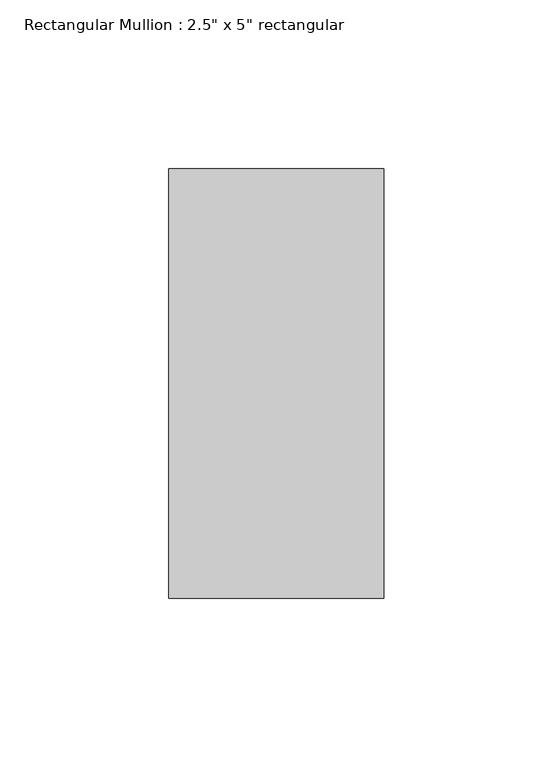
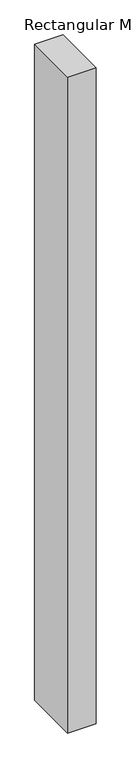
"""IFC4 building model written with IfcOpenShell, lengths in millimetres: member geometry."""

from ifc_helpers import new_model, si_unit, frame, origin, place, context, project, spatial, polyline, outline, extrude, source, transform, mapped, element, save


def member_b50ca06a(model_context):
    return source(origin(), model_context, "Body", "SweptSolid", [
        extrude(outline(polyline([(0.0, 63.5), (0.0, -63.5), (-63.5, -63.5), (-63.5, 63.5), (0.0, 63.5)])), frame((0.0, 0.0, -1544.4066766), z_axis=(0.0, 0.0, 1.0), x_axis=(1.0, 0.0, 0.0)), (0.0, 0.0, 1.0), 1544.4066766),
    ])


if __name__ == "__main__":
    model = new_model("IFC4")
    model_context = context("Model", 3, world=origin())
    ifc_project = project(units=[si_unit("LENGTHUNIT", "METRE", prefix="MILLI")], contexts=[model_context])
    site = spatial("IfcSite", under=ifc_project)
    building = spatial("IfcBuilding", under=site)
    placement = place(None, origin())
    member_shape = member_b50ca06a(model_context)
    element("IfcMember", 1, ObjectType="Rectangular Mullion : 2.5\" x 5\" rectangular", at=placement, inside=building, context=model_context, shape_type="MappedRepresentation", body=[
        mapped(member_shape, transform((0.0, 0.0, 0.0), x_axis=(1.0, 0.0, 0.0), y_axis=(0.0, 1.0, 0.0), z_axis=(0.0, 0.0, 1.0))),
    ])
    save(model, "model.ifc")

# Revit data of these elements
# Type "Rectangular Mullion : 2.5\" x 5\" rectangular"
#   built-in parameter 1007304 = 0.416667 (stored number, unit not read)
#   built-in parameter 1007301 = 0.104167 (stored number, unit not read)
#   built-in parameter 1007300 = 0.104167 (stored number, unit not read)
# Element 1 (IfcMember, "Rectangular Mullion : 2.5\" x 5\" rectangular")
#   Materials on its faces: "Aluminum"
# Materials
#   "Aluminum": class "Metal", colour RGB 247 247 247, transparency 0, Description = "Aluminum 6061", Cost = 0
